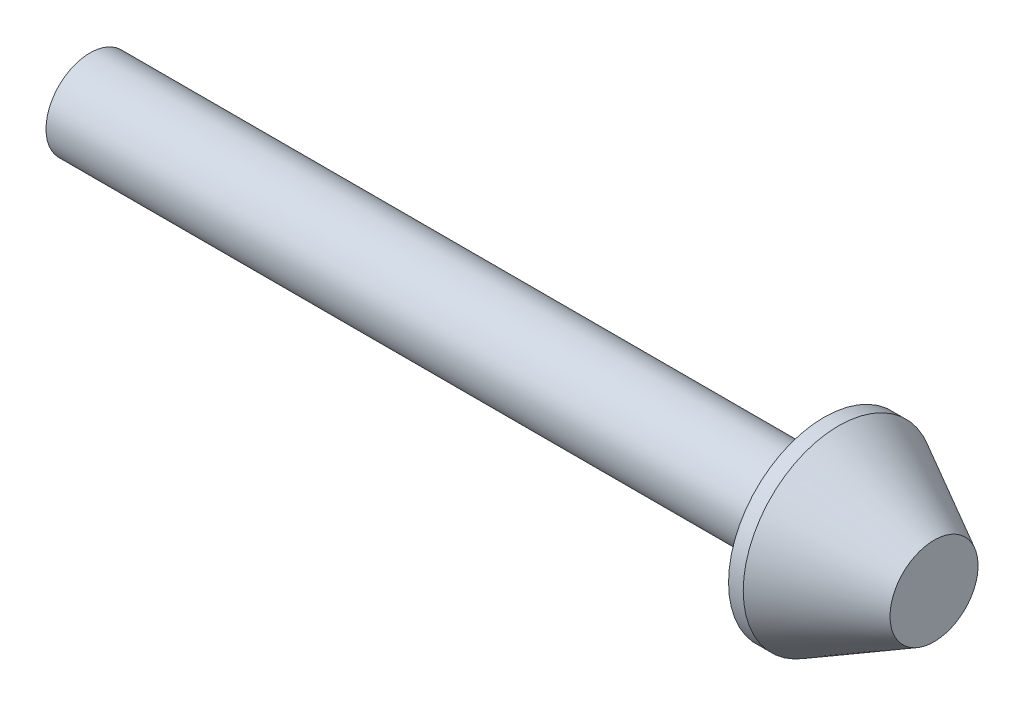
SolidWorks part; units mm, degrees
material "Plain Carbon Steel"
ref_plane "Front Plane" through (0, 0, 0) normal (0, 0, 1) x (1, 0, 0)
ref_plane "Top Plane" through (0, 0, 0) normal (0, 1, 0) x (1, 0, 0)
ref_plane "Right Plane" through (0, 0, 0) normal (1, 0, 0) x (0, 0, -1)
sketch "Rod Profile Sketch" plane through (0, 0, 0) normal (0, 0, 1) x (1, 0, 0)
  line L0 (0, 0) -> (115, 0)
  line L1 (115, 0) -> (115, 6)
  line L2 (115, 6) -> (102, 13)
  line L3 (102, 13) -> (100, 13)
  line L4 (100, 13) -> (100, 6)
  line L5 (100, 6) -> (0, 6)
  line L6 (0, 6) -> (0, 0)
  point P3 (101, 13)
  dimension "D1" = 100
  dimension "D2" = 2
  dimension "D3" = 6
  dimension "D4" = 6
  dimension "D5" = 115
  dimension "D6" = 13
revolve "Rod Body Revolve" add sketch "Rod Profile Sketch" angle 360 about L0
